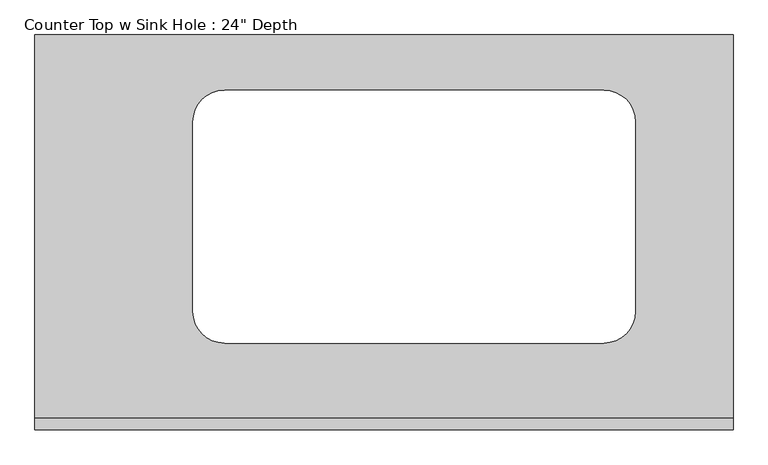
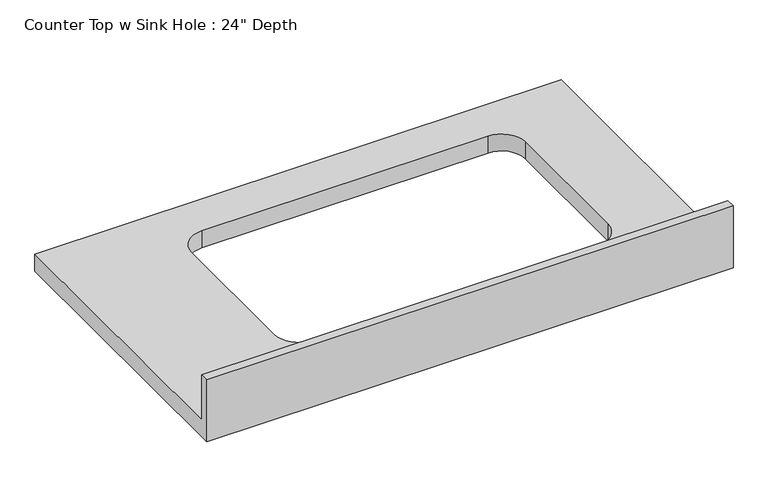
"""IFC4 building model written with IfcOpenShell, lengths in millimetres: furniture geometry."""

from ifc_helpers import new_model, si_unit, frame, origin, place, context, project, spatial, polyline, circle_curve, source, transform, mapped, element, save
from ifc_brep_helpers import plane_surface, revolved_surface, advanced_brep


def furniture_dd44345b(model_context):
    return source(origin(), model_context, "Body", "AdvancedBrep", [
        advanced_brep(
        [(-1200.4622951, 635.0, 914.4), (-1200.4622951, 19.05, 914.4), (-78.1397312, 19.05, 914.4), (-78.1397312, 635.0, 914.4), (-895.6622951, 139.7, 914.4), (-946.4622951, 190.5, 914.4), (-946.4622951, 495.3, 914.4), (-895.6622951, 546.1, 914.4), (-286.0622951, 546.1, 914.4), (-235.2622951, 495.3, 914.4), (-235.2622951, 190.5, 914.4), (-286.0622951, 139.7, 914.4), (-78.1397312, 0.0, 876.3), (-1200.4622951, 0.0, 876.3), (-1200.4622951, 635.0, 876.3), (-78.1397312, 635.0, 876.3), (-286.0622951, 139.7, 876.3), (-235.2622951, 190.5, 876.3), (-235.2622951, 495.3, 876.3), (-286.0622951, 546.1, 876.3), (-895.6622951, 546.1, 876.3), (-946.4622951, 495.3, 876.3), (-946.4622951, 190.5, 876.3), (-895.6622951, 139.7, 876.3), (-78.1397312, 0.0, 1016.0), (-1200.4622951, 0.0, 1016.0), (-1200.4622951, 19.05, 1016.0), (-78.1397312, 19.05, 1016.0)],
        [
            (0, 1),
            (1, 2),
            (2, 3),
            (3, 0),
            (4, 5, circle_curve(frame((-895.6622951, 190.5, 914.4), z_axis=(0.0, 0.0, -1.0), x_axis=(1.0, 0.0, 0.0)), 50.8)),
            (5, 6),
            (6, 7, circle_curve(frame((-895.6622951, 495.3, 914.4), z_axis=(0.0, 0.0, -1.0), x_axis=(1.0, 0.0, 0.0)), 50.8)),
            (7, 8),
            (8, 9, circle_curve(frame((-286.0622951, 495.3, 914.4), z_axis=(0.0, 0.0, -1.0), x_axis=(1.0, 0.0, 0.0)), 50.8)),
            (9, 10),
            (10, 11, circle_curve(frame((-286.0622951, 190.5, 914.4), z_axis=(0.0, 0.0, -1.0), x_axis=(1.0, 0.0, 0.0)), 50.8)),
            (11, 4),
            (12, 13),
            (13, 14),
            (14, 15),
            (15, 12),
            (16, 17, circle_curve(frame((-286.0622951, 190.5, 876.3), z_axis=(0.0, 0.0, 1.0), x_axis=(1.0, 0.0, 0.0)), 50.8)),
            (17, 18),
            (18, 19, circle_curve(frame((-286.0622951, 495.3, 876.3), z_axis=(0.0, 0.0, 1.0), x_axis=(1.0, 0.0, 0.0)), 50.8)),
            (19, 20),
            (20, 21, circle_curve(frame((-895.6622951, 495.3, 876.3), z_axis=(0.0, 0.0, 1.0), x_axis=(1.0, 0.0, 0.0)), 50.8)),
            (21, 22),
            (22, 23, circle_curve(frame((-895.6622951, 190.5, 876.3), z_axis=(0.0, 0.0, 1.0), x_axis=(1.0, 0.0, 0.0)), 50.8)),
            (23, 16),
            (12, 24),
            (24, 25),
            (25, 13),
            (25, 26),
            (26, 1),
            (0, 14),
            (3, 15),
            (2, 27),
            (27, 24),
            (27, 26),
            (11, 16),
            (23, 4),
            (22, 5),
            (21, 6),
            (20, 7),
            (19, 8),
            (18, 9),
            (17, 10),
        ],
        [
            plane_surface(frame((-1200.4622951, 0.0, 914.4), z_axis=(0.0, 0.0, 1.0), x_axis=(-1.0, 0.0, 0.0))),
            plane_surface(frame((-1200.4622951, 0.0, 876.3), z_axis=(0.0, 0.0, -1.0), x_axis=(1.0, 0.0, 0.0))),
            plane_surface(frame((-78.1397312, 0.0, 914.4), z_axis=(0.0, -1.0, 0.0), x_axis=(0.0, 0.0, -1.0))),
            plane_surface(frame((-1200.4622951, 0.0, 914.4), z_axis=(-1.0, 0.0, 0.0), x_axis=(0.0, 0.0, -1.0))),
            plane_surface(frame((-1200.4622951, 635.0, 914.4), z_axis=(0.0, 1.0, 0.0), x_axis=(0.0, 0.0, -1.0))),
            plane_surface(frame((-78.1397312, 635.0, 914.4), z_axis=(1.0, 0.0, 0.0), x_axis=(0.0, 0.0, -1.0))),
            plane_surface(frame((-1200.4622951, 0.0, 1016.0), z_axis=(0.0, 0.0, 1.0), x_axis=(0.0, 1.0, 0.0))),
            plane_surface(frame((-1200.4622951, 19.05, 1016.0), z_axis=(0.0, 1.0, 0.0), x_axis=(0.0, 0.0, -1.0))),
            plane_surface(frame((-286.0622951, 139.7, 914.4), z_axis=(0.0, 1.0, 0.0), x_axis=(0.0, 0.0, -1.0))),
            revolved_surface(polyline([(-844.8622951000001, 190.5, 914.4), (-844.8622951000001, 190.5, 876.3)]), (-895.6622951, 190.5, 876.3), (0.0, 0.0, 1.0)),
            plane_surface(frame((-946.4622951, 190.5, 914.4), z_axis=(1.0, 0.0, 0.0), x_axis=(0.0, 0.0, -1.0))),
            revolved_surface(polyline([(-844.8622951000001, 495.3, 914.4), (-844.8622951000001, 495.3, 876.3)]), (-895.6622951, 495.3, 876.3), (0.0, 0.0, 1.0)),
            plane_surface(frame((-895.6622951, 546.1, 914.4), z_axis=(0.0, -1.0, 0.0), x_axis=(0.0, 0.0, -1.0))),
            revolved_surface(polyline([(-235.26229509999996, 495.3, 914.4), (-235.26229509999996, 495.3, 876.3)]), (-286.0622951, 495.3, 876.3), (0.0, 0.0, 1.0)),
            plane_surface(frame((-235.2622951, 495.3, 914.4), z_axis=(-1.0, 0.0, 0.0), x_axis=(0.0, 0.0, -1.0))),
            revolved_surface(polyline([(-235.26229509999996, 190.5, 914.4), (-235.26229509999996, 190.5, 876.3)]), (-286.0622951, 190.5, 876.3), (0.0, 0.0, 1.0)),
        ],
        [
            (0, [[1, 2, 3, 4], [5, 6, 7, 8, 9, 10, 11, 12]]),
            (1, [[13, 14, 15, 16], [17, 18, 19, 20, 21, 22, 23, 24]]),
            (2, [[25, 26, 27, -13]]),
            (3, [[-27, 28, 29, -1, 30, -14]]),
            (4, [[31, -15, -30, -4]]),
            (5, [[-31, -3, 32, 33, -25, -16]]),
            (6, [[-26, -33, 34, -28]]),
            (7, [[-32, -2, -29, -34]]),
            (8, [[-12, 35, -24, 36]]),
            (9, [[-23, 37, -5, -36]]),
            (10, [[-22, 38, -6, -37]]),
            (11, [[-21, 39, -7, -38]]),
            (12, [[-20, 40, -8, -39]]),
            (13, [[-19, 41, -9, -40]]),
            (14, [[-18, 42, -10, -41]]),
            (15, [[-11, -42, -17, -35]]),
        ],
    ),
    ])


if __name__ == "__main__":
    model = new_model("IFC4")
    model_context = context("Model", 3, world=origin())
    ifc_project = project(units=[si_unit("LENGTHUNIT", "METRE", prefix="MILLI")], contexts=[model_context])
    site = spatial("IfcSite", under=ifc_project)
    building = spatial("IfcBuilding", under=site)
    placement = place(None, origin())
    furniture_shape = furniture_dd44345b(model_context)
    element("IfcFurniture", 1, ObjectType="Counter Top w Sink Hole : 24\" Depth", at=placement, inside=building, context=model_context, shape_type="MappedRepresentation", body=[
        mapped(furniture_shape, transform((0.0, 0.0, 0.0), x_axis=(1.0, 0.0, 0.0), y_axis=(0.0, 1.0, 0.0), z_axis=(0.0, 0.0, 1.0))),
    ])
    save(model, "model.ifc")

# Revit data of these elements
# Type "Counter Top w Sink Hole : 24\" Depth"
#   Assembly Code = "C1030400"
#   Counter Thickness = 0' - 1 1/2"
#   Depth = 2' - 1"
#   Height = 3' - 0"
#   Length [instance default] = 8' - 0"
#   Sink Location [instance default] = 2' - 0"
#   Sink Location To Wall [instance default] = 0' - 6"
#   Sink Opening Depth [instance default] = 1' - 3"
#   Sink Opening Width [instance default] = 2' - 3"
#   Counter Top Material = none
#   Default Elevation = 0
# Element 1 (IfcFurniture, "Counter Top w Sink Hole : 24\" Depth")
#   Length = 3' - 8.18593"
#   Materials on its faces: "Counter Top"
# Materials
#   "Counter Top": class "Wood", colour RGB 226 177 128, transparency 0
